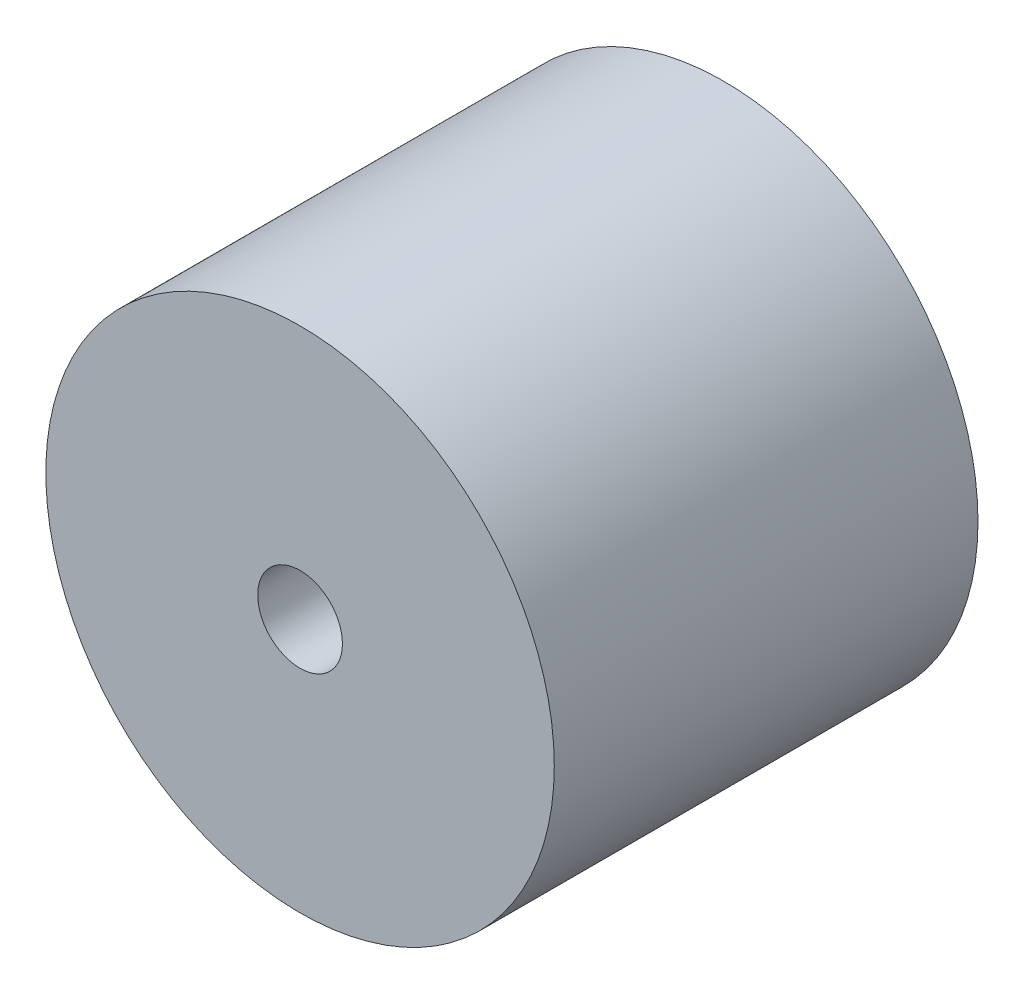
from build123d import *

# Parameters (mm, degrees)
BUSHING_PROFILE_36_6_R   = 18
BUSHING_PROFILE_36_6_R_2 = 3
BUSHING_BODY_L30_DEPTH   = 15


with BuildPart() as part:
    # Bushing Profile Ø36-Ø6 → Bushing Body L30 (new, symmetric)
    with BuildSketch(Plane.XY):
        Circle(BUSHING_PROFILE_36_6_R)
        Circle(BUSHING_PROFILE_36_6_R_2, mode=Mode.SUBTRACT)
    extrude(amount=BUSHING_BODY_L30_DEPTH, both=True)


solid = part.part
